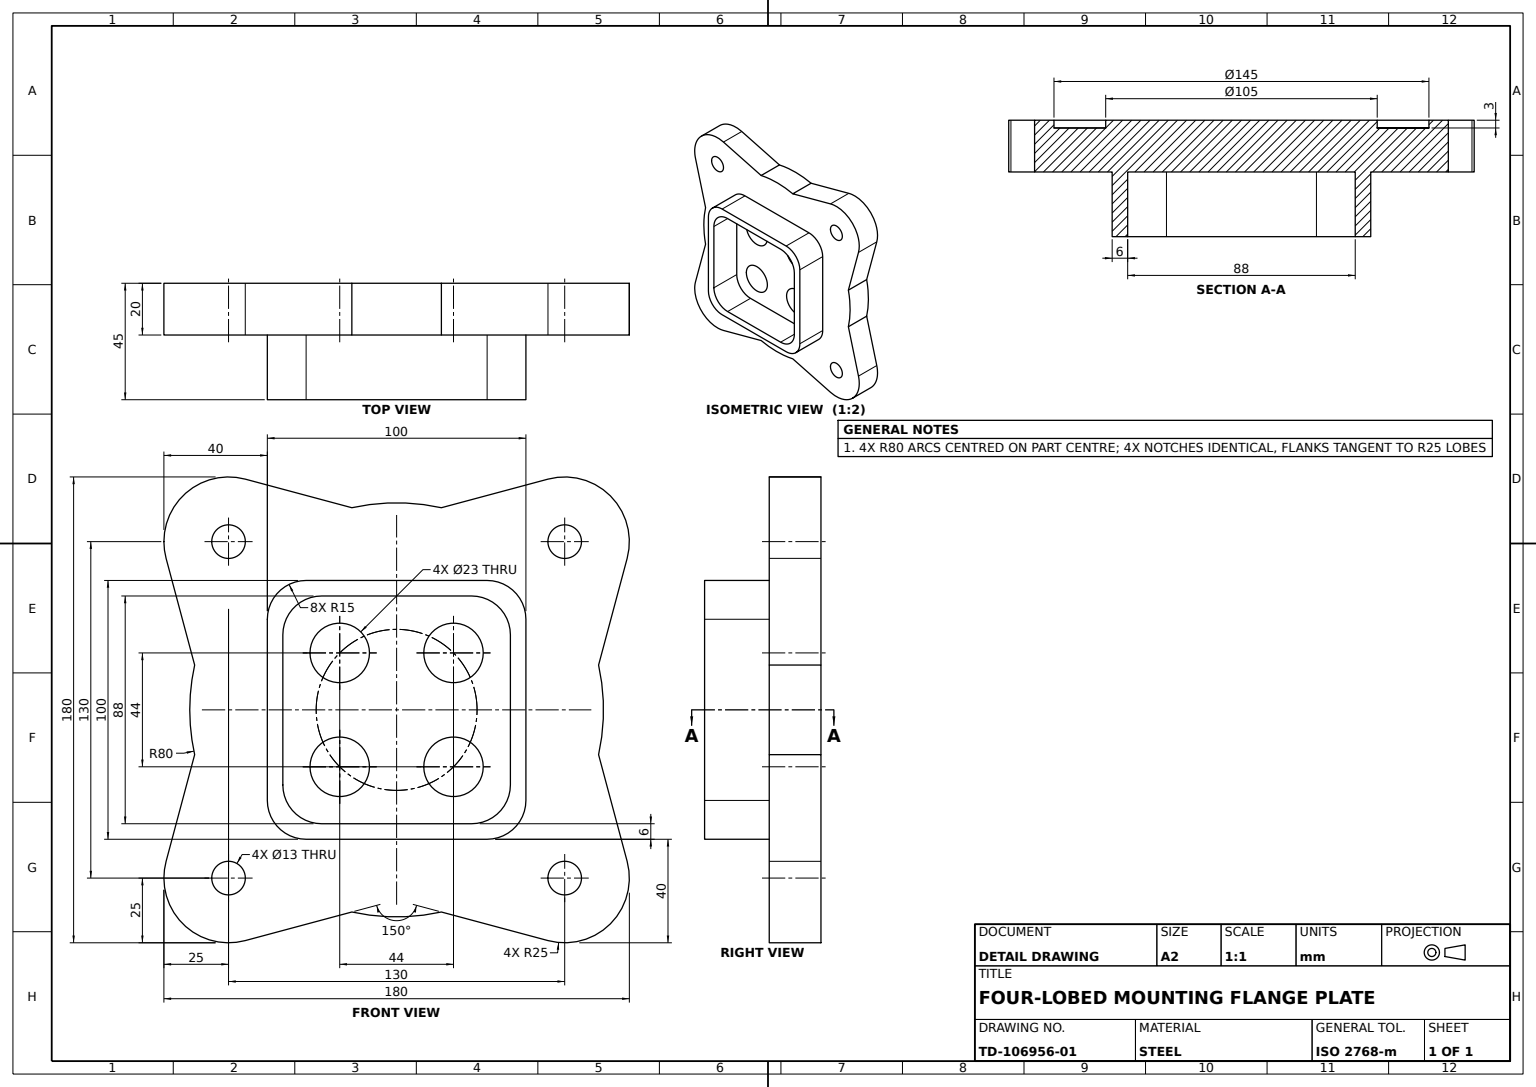
from build123d import *

# Parameters (mm, degrees)
FLANGE_PROFILE_SKETCH_R   = 6.5
FLANGE_PLATE_20MM_DEPTH   = 20
FLANGE_PROFILE_SKETCH_R_2 = 11.5
FLANGE_PLATE_20MM_2_DEPTH = 20
SQUARE_BOSS_45MM_DEPTH    = 45
BOSS_POCKET_SKETCH_R      = 72.5
BOSS_POCKET_SKETCH_R_2    = 52.5
BOSS_POCKET_CUT_DEPTH     = 3


with BuildPart() as part:
    # Flange Profile Sketch → Flange Plate 20mm (new body)
    with BuildSketch(Plane.XY):
        with BuildLine():
            Line((-89.148145657, 58.529523872), (-78.104184034, 17.312897978))
            ThreePointArc((-78.104184034, 17.312897978), (-80, 0), (-78.104184034, -17.312897978))
            Line((-78.104184034, -17.312897978), (-89.148145657, -58.529523872))
            ThreePointArc((-89.148145657, -58.529523872), (-82.677671147, -82.677667913), (-58.52952829, -89.148146841))
            Line((-58.52952829, -89.148146841), (-17.312897978, -78.104184034))
            ThreePointArc((-17.312897978, -78.104184034), (-8.453e-06, -80), (17.312881472, -78.104187693))
            Line((17.312881472, -78.104187693), (58.52952829, -89.148146841))
            ThreePointArc((58.52952829, -89.148146841), (82.677672617, -82.677669383), (89.148145657, -58.529523872))
            Line((89.148145657, -58.529523872), (78.104184034, -17.312897978))
            ThreePointArc((78.104184034, -17.312897978), (80, 0), (78.104184034, 17.312897978))
            Line((78.104184034, 17.312897978), (89.148145657, 58.529523872))
            ThreePointArc((89.148145657, 58.529523872), (82.67767031, 82.677667076), (58.52952829, 89.148146841))
            Line((58.52952829, 89.148146841), (17.312897978, 78.104184034))
            ThreePointArc((17.312897978, 78.104184034), (8.453e-06, 80), (-17.312881472, 78.104187693))
            Line((-17.312881472, 78.104187693), (-58.52952829, 89.148146841))
            ThreePointArc((-58.52952829, 89.148146841), (-82.677671147, 82.677667913), (-89.148145657, 58.529523872))
        make_face()
        with Locations((-65, -65)):
            Circle(FLANGE_PROFILE_SKETCH_R, mode=Mode.SUBTRACT)
        with Locations((65.00000294, -65.00000294)):
            Circle(FLANGE_PROFILE_SKETCH_R, mode=Mode.SUBTRACT)
        with Locations((64.999998327, 64.999998327)):
            Circle(FLANGE_PROFILE_SKETCH_R, mode=Mode.SUBTRACT)
        with Locations((-65, 65)):
            Circle(FLANGE_PROFILE_SKETCH_R, mode=Mode.SUBTRACT)
        with BuildLine():
            Line((-50, -35), (-50, 35))
            ThreePointArc((-50, 35), (-45.606601718, 45.606601718), (-35, 50))
            Line((-35, 50), (35, 50))
            ThreePointArc((35, 50), (45.606601718, 45.606601718), (50, 35))
            Line((50, 35), (50, -35))
            ThreePointArc((50, -35), (45.606601718, -45.606601718), (35, -50))
            Line((35, -50), (-35, -50))
            ThreePointArc((-35, -50), (-45.606601718, -45.606601718), (-50, -35))
        make_face(mode=Mode.SUBTRACT)
    extrude(amount=FLANGE_PLATE_20MM_DEPTH)



with BuildPart() as body_2:
    # Flange Profile Sketch → Flange Plate 20mm 2 (new body)
    with BuildSketch(Plane.XY):
        with BuildLine():
            ThreePointArc((-44, 29), (-39.606601718, 39.606601718), (-29, 44))
            Line((-29, 44), (29, 44))
            ThreePointArc((29, 44), (39.606601718, 39.606601718), (44, 29))
            Line((44, 29), (44, -29))
            ThreePointArc((44, -29), (39.606601718, -39.606601718), (29, -44))
            Line((29, -44), (-29, -44))
            ThreePointArc((-29, -44), (-39.606601718, -39.606601718), (-44, -29))
            Line((-44, -29), (-44, 29))
        make_face()
        with Locations((-22, 22)):
            Circle(FLANGE_PROFILE_SKETCH_R_2, mode=Mode.SUBTRACT)
        with Locations((22, 22)):
            Circle(FLANGE_PROFILE_SKETCH_R_2, mode=Mode.SUBTRACT)
        with Locations((22, -22)):
            Circle(FLANGE_PROFILE_SKETCH_R_2, mode=Mode.SUBTRACT)
        with Locations((-22, -22)):
            Circle(FLANGE_PROFILE_SKETCH_R_2, mode=Mode.SUBTRACT)
    extrude(amount=FLANGE_PLATE_20MM_2_DEPTH)


with BuildPart() as part_1:
    add(part.part)

    add(body_2.part)  # Square Boss 45mm merges body 2
    # Sketch2_6 → Square Boss 45mm (add)
    with BuildSketch(Plane.XY):
        with BuildLine():
            ThreePointArc((-50, 35), (-45.606601718, 45.606601718), (-35, 50))
            Line((-35, 50), (35, 50))
            ThreePointArc((35, 50), (45.606601718, 45.606601718), (50, 35))
            Line((50, 35), (50, -35))
            ThreePointArc((50, -35), (45.606601718, -45.606601718), (35, -50))
            Line((35, -50), (-35, -50))
            ThreePointArc((-35, -50), (-45.606601718, -45.606601718), (-50, -35))
            Line((-50, -35), (-50, 35))
        make_face()
        with BuildLine():
            Line((-44, -29), (-44, 29))
            ThreePointArc((-44, 29), (-39.606601718, 39.606601718), (-29, 44))
            Line((-29, 44), (29, 44))
            ThreePointArc((29, 44), (39.606601718, 39.606601718), (44, 29))
            Line((44, 29), (44, -29))
            ThreePointArc((44, -29), (39.606601718, -39.606601718), (29, -44))
            Line((29, -44), (-29, -44))
            ThreePointArc((-29, -44), (-39.606601718, -39.606601718), (-44, -29))
        make_face(mode=Mode.SUBTRACT)
    extrude(amount=SQUARE_BOSS_45MM_DEPTH)

    # Boss Pocket Sketch → Boss Pocket Cut (cut)
    with BuildSketch(Plane(origin=(0, 0, 0), x_dir=(-1, 0, 0), z_dir=(0, 0, -1))):
        Circle(BOSS_POCKET_SKETCH_R)
        Circle(BOSS_POCKET_SKETCH_R_2, mode=Mode.SUBTRACT)
    extrude(amount=-BOSS_POCKET_CUT_DEPTH, mode=Mode.SUBTRACT)


solid = part_1.part
